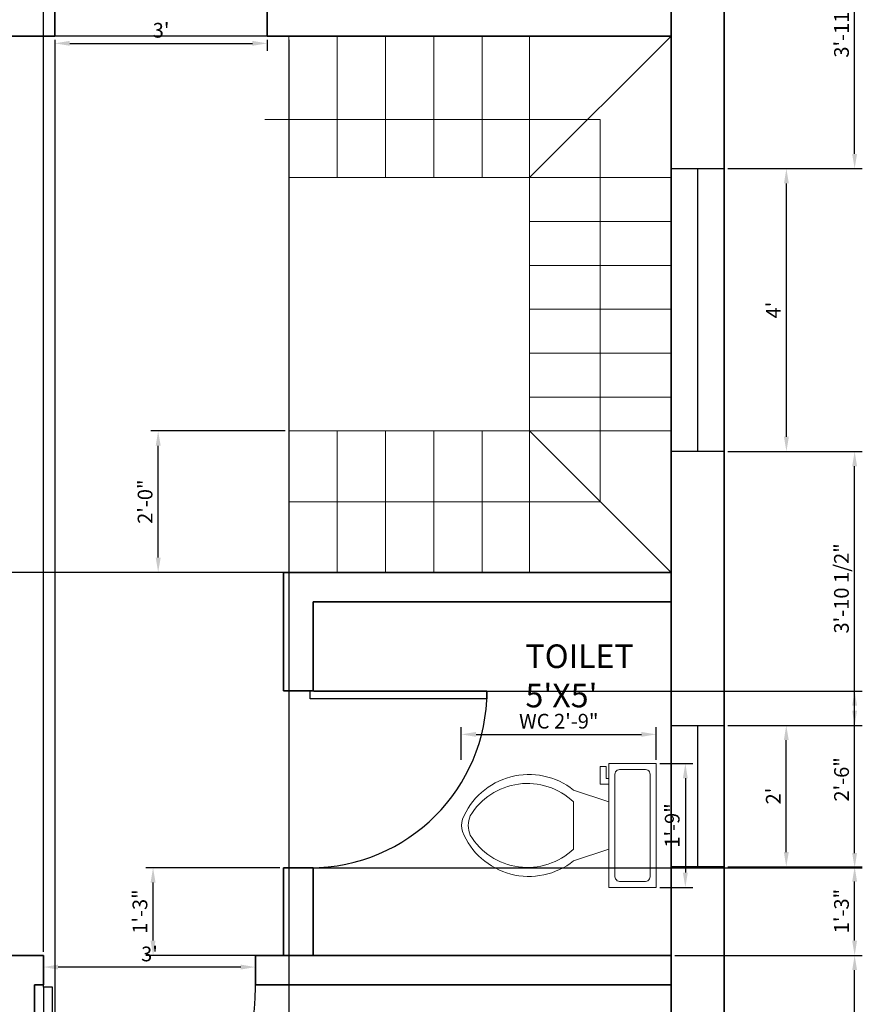
# Model space of a CAD drawing. Units: inches. Extents: x 2459 to 2755, y 1300 to 1776.
# Tile 3 of 4: x 2606 to 2750, y 1450 to 1617. Entities that reach past the tile are written whole.
import ezdxf

# ---------------------------------------------------------------- set-up
doc = ezdxf.new("R2010")
doc.units = ezdxf.units.IN
for name, color, linetype, lineweight in [('A-AREA-IDEN', 3, 'Continuous', 25), ('A-FLOR-FIXT', 8, 'Continuous', 18), ('A-FLOR-STRS', 7, 'Continuous', 18), ('A-WALL', 7, 'Continuous', 35), ('DIM', 4, 'Continuous', 18), ('DOOR', 20, 'Continuous', 25), ('WIN', 2, 'Continuous', 25)]:
    doc.layers.add(name, color=color, linetype=linetype, lineweight=lineweight)
doc.styles.get("Standard").update_dxf_attribs({"font": 'arial.ttf'})
doc.dimstyles.new('ISO-25', dxfattribs={"dimtxt": 2.5, "dimasz": 2.5, "dimexe": 1.25, "dimexo": 0.625, "dimtad": 1, "dimlunit": 3, "dimtxsty": 'Standard', "dimcen": 2.5, "dimadec": 0, "dimazin": 0, "dimtfac": 1, "dimtmove": 0, "dimatfit": 3, "dimfxl": 1, "dimarcsym": 0})

# ---------------------------------------------------------------- blocks, each defined once
blk = doc.blocks.new('*U2')
for p, q in [((0, 0), (0, -6)), ((40, 0), (40, -6))]:
    blk.add_line(p, q)
blk.add_lwpolyline([(0, 0), (0, 40), (1.75, 40), (1.75, 0)], close=True)
blk.add_arc((0, 0), 40, 0, 90)
blk = doc.blocks.new('*U5')
for p, q in [((0, 0), (0, 6)), ((40, 0), (40, 6))]:
    blk.add_line(p, q)
blk.add_lwpolyline([(0, 0), (0, -40), (1.75, -40), (1.75, 0)], close=True)
blk.add_arc((0, 0), 40, 270, 0)
blk = doc.blocks.new('Toilet - top')
for p, q in [((9.5, -6), (9.5, -2)), ((-8, -8.5), (-8, -8)), ((-7, -8), (-7, -9.5)), ((-4, -8), (-6, -14)), ((4, -8), (6, -14)), ((-10, -8.5), (-8, -8.5)), ((-10, -9.5), (-10, -8.5)), ((-7, -9.5), (-10, -9.5)), ((4, -14), (-4, -14))]:
    blk.add_line(p, q)
blk.add_lwpolyline([(10.5, -8), (10.5, 0), (-10.5, 0), (-10.5, -8)], close=True)
for points in [[(8.5, -1), (-8.5, -1)], [(-9.5, -2), (-9.5, -6)], [(-8.5, -7), (8.5, -7)]]:
    blk.add_lwpolyline(points)
for centre, radius, start, end in [((-8.62, -1.88), 0.884, 81.8699, 188.1301), ((8.62, -1.88), 0.884, 351.8699, 98.1301), ((-8.62, -6.12), 0.884, 171.8699, 278.1301), ((8.62, -6.12), 0.884, 261.8699, 8.1301), ((3.52, -21.58), 12.17, 141.4691, 247.9714), ((4.2, -21.82), 11.33, 136.3677, 238.9468), ((-3.52, -21.58), 12.17, 292.0284, 38.5307), ((-4.2, -21.82), 11.33, 301.053, 43.6321), ((0, -27.88), 4, 245.7318, 294.2682), ((0, -29), 4, 254.8605, 285.1395)]:
    blk.add_arc(centre, radius, start, end)
blk = doc.blocks.new('*D23')
at = {"layer": 'Defpoints', "color": 0, "transparency": 16777216}
for p in [(2612.48, 1614.32), (2648.48, 1614.32), (2648.48, 1613.1)]:
    blk.add_point(p, dxfattribs=at)
at = {"layer": 'DIM', "color": 0, "lineweight": -2, "transparency": 16777216}
for p, q in [((2612.48, 1613.69), (2612.48, 1611.85)), ((2614.98, 1613.1), (2645.98, 1613.1)), ((2648.48, 1613.69), (2648.48, 1611.85))]:
    blk.add_line(p, q, dxfattribs=at)
at = {"layer": 'DIM', "color": 0, "transparency": 16777216}
for points in [[(2614.98, 1613.52), (2614.98, 1612.69), (2612.48, 1613.1)], [(2645.98, 1613.52), (2645.98, 1612.69), (2648.48, 1613.1)]]:
    blk.add_solid(points, dxfattribs=at)
at = {"layer": 'DIM', "color": 0, "transparency": 16777216, "insert": (2630.48, 1615), "char_height": 2.5, "attachment_point": 5}
blk.add_mtext("3'", dxfattribs=at)
blk = doc.blocks.new('*D27')
at = {"layer": 'Defpoints', "color": 0, "transparency": 16777216}
for p in [(2726, 1497.36), (2736.55, 1497.36), (2726, 1473.36)]:
    blk.add_point(p, dxfattribs=at)
at = {"layer": 'DIM', "color": 0, "lineweight": -2, "transparency": 16777216}
for p, q in [((2726.62, 1497.36), (2737.8, 1497.36)), ((2736.55, 1475.86), (2736.55, 1494.86)), ((2726.62, 1473.36), (2737.8, 1473.36))]:
    blk.add_line(p, q, dxfattribs=at)
at = {"layer": 'DIM', "color": 0, "transparency": 16777216}
for points in [[(2736.14, 1494.86), (2736.97, 1494.86), (2736.55, 1497.36)], [(2736.14, 1475.86), (2736.97, 1475.86), (2736.55, 1473.36)]]:
    blk.add_solid(points, dxfattribs=at)
at = {"layer": 'DIM', "color": 0, "transparency": 16777216, "insert": (2734.67, 1485.36), "char_height": 2.5, "attachment_point": 5, "rotation": 90}
blk.add_mtext("2'", dxfattribs=at)
blk = doc.blocks.new('*D28')
at = {"layer": 'Defpoints', "color": 0, "transparency": 16777216}
for p in [(2726, 1591.84), (2736.57, 1591.84), (2726, 1543.84)]:
    blk.add_point(p, dxfattribs=at)
at = {"layer": 'DIM', "color": 0, "lineweight": -2, "transparency": 16777216}
for p, q in [((2726.62, 1591.84), (2737.82, 1591.84)), ((2736.57, 1546.34), (2736.57, 1589.34)), ((2726.62, 1543.84), (2737.82, 1543.84))]:
    blk.add_line(p, q, dxfattribs=at)
at = {"layer": 'DIM', "color": 0, "transparency": 16777216}
for points in [[(2736.16, 1589.34), (2736.99, 1589.34), (2736.57, 1591.84)], [(2736.16, 1546.34), (2736.99, 1546.34), (2736.57, 1543.84)]]:
    blk.add_solid(points, dxfattribs=at)
at = {"layer": 'DIM', "color": 0, "transparency": 16777216, "insert": (2734.7, 1567.84), "char_height": 2.5, "attachment_point": 5, "rotation": 90}
blk.add_mtext("4'", dxfattribs=at)
blk = doc.blocks.new('*D32')
at = {"layer": 'Defpoints', "color": 0, "transparency": 16777216}
for p in [(2610.51, 1458.32), (2646.51, 1458.32), (2610.51, 1456.34)]:
    blk.add_point(p, dxfattribs=at)
at = {"layer": 'DIM', "color": 0, "lineweight": -2, "transparency": 16777216}
for p, q in [((2610.51, 1457.69), (2610.51, 1455.09)), ((2646.51, 1457.69), (2646.51, 1455.09)), ((2644.01, 1456.34), (2613.01, 1456.34))]:
    blk.add_line(p, q, dxfattribs=at)
at = {"layer": 'DIM', "color": 0, "transparency": 16777216}
for points in [[(2613.01, 1456.75), (2613.01, 1455.92), (2610.51, 1456.34)], [(2644.01, 1456.75), (2644.01, 1455.92), (2646.51, 1456.34)]]:
    blk.add_solid(points, dxfattribs=at)
at = {"layer": 'DIM', "color": 0, "transparency": 16777216, "insert": (2628.51, 1458.24), "char_height": 2.5, "attachment_point": 5}
blk.add_mtext("3'", dxfattribs=at)
blk = doc.blocks.new('WIN-48IN')
blk.add_line((4.5, 48), (4.5, 0))
blk.add_lwpolyline([(0, 48), (9, 48), (9, 0), (0, 0)], close=True)
blk = doc.blocks.new('WIN-24IN')
blk.add_line((4.5, 24), (4.5, 0))
blk.add_lwpolyline([(0, 24), (9, 24), (9, 0), (0, 0)], close=True)
blk = doc.blocks.new('*D55')
at = {"layer": 'Defpoints', "color": 0, "transparency": 16777216}
for p in [(2714.47, 1495.83), (2681.42, 1490.87), (2714.47, 1490.87)]:
    blk.add_point(p, dxfattribs=at)
at = {"layer": 'DIM', "color": 0, "lineweight": -2, "transparency": 16777216}
for p, q in [((2681.42, 1491.49), (2681.42, 1497.08)), ((2683.92, 1495.83), (2711.97, 1495.83)), ((2714.47, 1491.49), (2714.47, 1497.08))]:
    blk.add_line(p, q, dxfattribs=at)
at = {"layer": 'DIM', "color": 0, "transparency": 16777216}
for points in [[(2683.92, 1496.24), (2683.92, 1495.41), (2681.42, 1495.83)], [(2711.97, 1496.24), (2711.97, 1495.41), (2714.47, 1495.83)]]:
    blk.add_solid(points, dxfattribs=at)
at = {"layer": 'DIM', "color": 0, "transparency": 16777216, "insert": (2697.95, 1497.74), "char_height": 2.5, "attachment_point": 5}
blk.add_mtext('WC 2\'-9"', dxfattribs=at)
blk = doc.blocks.new('*D56')
at = {"layer": 'Defpoints', "color": 0, "transparency": 16777216}
for p in [(2714.47, 1490.87), (2714.47, 1469.87), (2719.43, 1469.87)]:
    blk.add_point(p, dxfattribs=at)
at = {"layer": 'DIM', "color": 0, "lineweight": -2, "transparency": 16777216}
for p, q in [((2715.09, 1490.87), (2720.68, 1490.87)), ((2719.43, 1488.37), (2719.43, 1472.37)), ((2715.09, 1469.87), (2720.68, 1469.87))]:
    blk.add_line(p, q, dxfattribs=at)
at = {"layer": 'DIM', "color": 0, "transparency": 16777216}
for points in [[(2719.01, 1488.37), (2719.84, 1488.37), (2719.43, 1490.87)], [(2719.01, 1472.37), (2719.84, 1472.37), (2719.43, 1469.87)]]:
    blk.add_solid(points, dxfattribs=at)
at = {"layer": 'DIM', "color": 0, "transparency": 16777216, "insert": (2717.52, 1480.37), "char_height": 2.5, "attachment_point": 5, "rotation": 90}
blk.add_mtext('1\'-9"', dxfattribs=at)
blk = doc.blocks.new('*D66')
at = {"layer": 'Defpoints', "color": 0, "transparency": 16777216}
for p in [(2717, 1458.32), (2748.15, 1458.32), (2726, 1423.98)]:
    blk.add_point(p, dxfattribs=at)
at = {"layer": 'DIM', "color": 0, "lineweight": -2, "transparency": 16777216}
for p, q in [((2717.62, 1458.32), (2749.4, 1458.32)), ((2748.15, 1426.48), (2748.15, 1455.82)), ((2726.62, 1423.98), (2749.4, 1423.98))]:
    blk.add_line(p, q, dxfattribs=at)
at = {"layer": 'DIM', "color": 0, "transparency": 16777216}
for points in [[(2747.73, 1455.82), (2748.56, 1455.82), (2748.15, 1458.32)], [(2747.73, 1426.48), (2748.56, 1426.48), (2748.15, 1423.98)]]:
    blk.add_solid(points, dxfattribs=at)
at = {"layer": 'DIM', "color": 0, "transparency": 16777216, "insert": (2746.23, 1441.15), "char_height": 2.5, "attachment_point": 5, "rotation": 90}
blk.add_mtext('2\'-10 1/2"', dxfattribs=at)
blk = doc.blocks.new('*D67')
at = {"layer": 'Defpoints', "color": 0, "transparency": 16777216}
for p in [(2726, 1473.36), (2748.15, 1473.36), (2717, 1458.32)]:
    blk.add_point(p, dxfattribs=at)
at = {"layer": 'DIM', "color": 0, "lineweight": -2, "transparency": 16777216}
for p, q in [((2726.62, 1473.36), (2749.4, 1473.36)), ((2748.15, 1460.82), (2748.15, 1470.86)), ((2717.62, 1458.32), (2749.4, 1458.32))]:
    blk.add_line(p, q, dxfattribs=at)
at = {"layer": 'DIM', "color": 0, "transparency": 16777216}
for points in [[(2747.73, 1470.86), (2748.56, 1470.86), (2748.15, 1473.36)], [(2747.73, 1460.82), (2748.56, 1460.82), (2748.15, 1458.32)]]:
    blk.add_solid(points, dxfattribs=at)
at = {"layer": 'DIM', "color": 0, "transparency": 16777216, "insert": (2746.24, 1465.84), "char_height": 2.5, "attachment_point": 5, "rotation": 90}
blk.add_mtext('1\'-3"', dxfattribs=at)
blk = doc.blocks.new('*D68')
at = {"layer": 'Defpoints', "color": 0, "transparency": 16777216}
for p in [(2726, 1543.84), (2748.15, 1543.84), (2726, 1497.36)]:
    blk.add_point(p, dxfattribs=at)
at = {"layer": 'DIM', "color": 0, "lineweight": -2, "transparency": 16777216}
for p, q in [((2726.62, 1543.84), (2749.4, 1543.84)), ((2748.15, 1499.86), (2748.15, 1541.34)), ((2726.62, 1497.36), (2749.4, 1497.36))]:
    blk.add_line(p, q, dxfattribs=at)
at = {"layer": 'DIM', "color": 0, "transparency": 16777216}
for points in [[(2747.73, 1541.34), (2748.56, 1541.34), (2748.15, 1543.84)], [(2747.73, 1499.86), (2748.56, 1499.86), (2748.15, 1497.36)]]:
    blk.add_solid(points, dxfattribs=at)
at = {"layer": 'DIM', "color": 0, "transparency": 16777216, "insert": (2746.23, 1520.6), "char_height": 2.5, "attachment_point": 5, "rotation": 90}
blk.add_mtext('3\'-10 1/2"', dxfattribs=at)
blk = doc.blocks.new('*D69')
at = {"layer": 'Defpoints', "color": 0, "transparency": 16777216}
for p in [(2726, 1638.95), (2748.15, 1638.95), (2726, 1591.84)]:
    blk.add_point(p, dxfattribs=at)
at = {"layer": 'DIM', "color": 0, "lineweight": -2, "transparency": 16777216}
for p, q in [((2726.62, 1638.95), (2749.4, 1638.95)), ((2748.15, 1594.34), (2748.15, 1636.45)), ((2726.62, 1591.84), (2749.4, 1591.84))]:
    blk.add_line(p, q, dxfattribs=at)
at = {"layer": 'DIM', "color": 0, "transparency": 16777216}
for points in [[(2747.73, 1636.45), (2748.56, 1636.45), (2748.15, 1638.95)], [(2747.73, 1594.34), (2748.56, 1594.34), (2748.15, 1591.84)]]:
    blk.add_solid(points, dxfattribs=at)
at = {"layer": 'DIM', "color": 0, "transparency": 16777216, "insert": (2746.24, 1615.39), "char_height": 2.5, "attachment_point": 5, "rotation": 90}
blk.add_mtext('3\'-11"', dxfattribs=at)
blk = doc.blocks.new('*D71')
at = {"layer": 'Defpoints', "color": 0, "transparency": 16777216}
for p in [(2655.77, 1503.19), (2748.15, 1503.19), (2655.77, 1473.19)]:
    blk.add_point(p, dxfattribs=at)
at = {"layer": 'DIM', "color": 0, "lineweight": -2, "transparency": 16777216}
for p, q in [((2656.39, 1503.19), (2749.4, 1503.19)), ((2748.15, 1475.69), (2748.15, 1500.69)), ((2656.39, 1473.19), (2749.4, 1473.19))]:
    blk.add_line(p, q, dxfattribs=at)
at = {"layer": 'DIM', "color": 0, "transparency": 16777216}
for points in [[(2747.73, 1500.69), (2748.56, 1500.69), (2748.15, 1503.19)], [(2747.73, 1475.69), (2748.56, 1475.69), (2748.15, 1473.19)]]:
    blk.add_solid(points, dxfattribs=at)
at = {"layer": 'DIM', "color": 0, "transparency": 16777216, "insert": (2746.25, 1488.19), "char_height": 2.5, "attachment_point": 5, "rotation": 90}
blk.add_mtext('2\'-6"', dxfattribs=at)
blk = doc.blocks.new('*D72')
at = {"layer": 'Defpoints', "color": 0, "transparency": 16777216}
for p in [(2652.14, 1614.32), (2717, 1614.32), (2717, 1302.17)]:
    blk.add_point(p, dxfattribs=at)
at = {"layer": 'DIM', "color": 0, "lineweight": -2, "transparency": 16777216}
for p, q in [((2652.14, 1613.69), (2652.14, 1300.92)), ((2717, 1613.69), (2717, 1300.92)), ((2654.64, 1302.17), (2714.5, 1302.17))]:
    blk.add_line(p, q, dxfattribs=at)
at = {"layer": 'DIM', "color": 0, "transparency": 16777216}
for points in [[(2654.64, 1302.58), (2654.64, 1301.75), (2652.14, 1302.17)], [(2714.5, 1302.58), (2714.5, 1301.75), (2717, 1302.17)]]:
    blk.add_solid(points, dxfattribs=at)
at = {"layer": 'DIM', "color": 0, "transparency": 16777216, "insert": (2684.57, 1304.06), "char_height": 2.5, "attachment_point": 5}
blk.add_mtext('5\'-5"', dxfattribs=at)
blk = doc.blocks.new('*D73')
at = {"layer": 'Defpoints', "color": 0, "transparency": 16777216}
for p in [(2464.85, 1614.32), (2652.14, 1614.32), (2652.14, 1523.32)]:
    blk.add_point(p, dxfattribs=at)
at = {"layer": 'DIM', "color": 0, "lineweight": -2, "transparency": 16777216}
for p, q in [((2651.52, 1614.32), (2463.6, 1614.32)), ((2464.85, 1525.82), (2464.85, 1611.82)), ((2651.52, 1523.32), (2463.6, 1523.32))]:
    blk.add_line(p, q, dxfattribs=at)
at = {"layer": 'DIM', "color": 0, "transparency": 16777216}
for points in [[(2464.43, 1611.82), (2465.26, 1611.82), (2464.85, 1614.32)], [(2464.43, 1525.82), (2465.26, 1525.82), (2464.85, 1523.32)]]:
    blk.add_solid(points, dxfattribs=at)
at = {"layer": 'DIM', "color": 0, "transparency": 16777216, "insert": (2462.97, 1568.82), "char_height": 2.5, "attachment_point": 5, "rotation": 90}
blk.add_mtext('7\'-7"', dxfattribs=at)
blk = doc.blocks.new('*D74')
at = {"layer": 'Defpoints', "color": 0, "transparency": 16777216}
for p in [(2629.99, 1547.32), (2652.14, 1547.32), (2652.14, 1523.32)]:
    blk.add_point(p, dxfattribs=at)
at = {"layer": 'DIM', "color": 0, "lineweight": -2, "transparency": 16777216}
for p, q in [((2651.52, 1547.32), (2628.74, 1547.32)), ((2629.99, 1525.82), (2629.99, 1544.82)), ((2651.52, 1523.32), (2628.74, 1523.32))]:
    blk.add_line(p, q, dxfattribs=at)
at = {"layer": 'DIM', "color": 0, "transparency": 16777216}
for points in [[(2629.57, 1544.82), (2630.41, 1544.82), (2629.99, 1547.32)], [(2629.57, 1525.82), (2630.41, 1525.82), (2629.99, 1523.32)]]:
    blk.add_solid(points, dxfattribs=at)
at = {"layer": 'DIM', "color": 0, "transparency": 16777216, "insert": (2628.09, 1535.32), "char_height": 2.5, "attachment_point": 5, "rotation": 90}
blk.add_mtext('2\'-0"', dxfattribs=at)
blk = doc.blocks.new('*D76')
at = {"layer": 'Defpoints', "color": 0, "transparency": 16777216}
for p in [(2597, 1614.32), (2612.48, 1614.32), (2612.48, 1302.17)]:
    blk.add_point(p, dxfattribs=at)
at = {"layer": 'DIM', "color": 0, "lineweight": -2, "transparency": 16777216}
for p, q in [((2597, 1613.69), (2597, 1300.92)), ((2612.48, 1613.69), (2612.48, 1300.92)), ((2599.5, 1302.17), (2609.98, 1302.17))]:
    blk.add_line(p, q, dxfattribs=at)
at = {"layer": 'DIM', "color": 0, "transparency": 16777216}
for points in [[(2599.5, 1302.58), (2599.5, 1301.75), (2597, 1302.17)], [(2609.98, 1302.58), (2609.98, 1301.75), (2612.48, 1302.17)]]:
    blk.add_solid(points, dxfattribs=at)
at = {"layer": 'DIM', "color": 0, "transparency": 16777216, "insert": (2604.74, 1304.09), "char_height": 2.5, "attachment_point": 5}
blk.add_mtext('1\'-3 1/2"', dxfattribs=at)
blk = doc.blocks.new('*D78')
at = {"layer": 'Defpoints', "color": 0, "transparency": 16777216}
for p in [(2610.51, 1770.47), (2590.97, 1458.32), (2610.51, 1458.32)]:
    blk.add_point(p, dxfattribs=at)
at = {"layer": 'DIM', "color": 0, "lineweight": -2, "transparency": 16777216}
for p, q in [((2590.97, 1458.94), (2590.97, 1771.72)), ((2610.51, 1458.94), (2610.51, 1771.72)), ((2593.47, 1770.47), (2608.01, 1770.47))]:
    blk.add_line(p, q, dxfattribs=at)
at = {"layer": 'DIM', "color": 0, "transparency": 16777216}
for points in [[(2593.47, 1770.88), (2593.47, 1770.05), (2590.97, 1770.47)], [(2608.01, 1770.88), (2608.01, 1770.05), (2610.51, 1770.47)]]:
    blk.add_solid(points, dxfattribs=at)
at = {"layer": 'DIM', "color": 0, "transparency": 16777216, "insert": (2600.74, 1772.38), "char_height": 2.5, "attachment_point": 5}
blk.add_mtext('1\'-7 1/2"', dxfattribs=at)
blk = doc.blocks.new('*D83')
at = {"layer": 'Defpoints', "color": 0, "transparency": 16777216}
for p in [(2629.12, 1473.19), (2651.27, 1473.19), (2651.27, 1458.32)]:
    blk.add_point(p, dxfattribs=at)
at = {"layer": 'DIM', "color": 0, "lineweight": -2, "transparency": 16777216}
for p, q in [((2650.64, 1473.19), (2627.87, 1473.19)), ((2629.12, 1460.82), (2629.12, 1470.69)), ((2650.64, 1458.32), (2627.87, 1458.32))]:
    blk.add_line(p, q, dxfattribs=at)
at = {"layer": 'DIM', "color": 0, "transparency": 16777216}
for points in [[(2628.7, 1470.69), (2629.54, 1470.69), (2629.12, 1473.19)], [(2628.7, 1460.82), (2629.54, 1460.82), (2629.12, 1458.32)]]:
    blk.add_solid(points, dxfattribs=at)
at = {"layer": 'DIM', "color": 0, "transparency": 16777216, "insert": (2627.22, 1465.76), "char_height": 2.5, "attachment_point": 5, "rotation": 90}
blk.add_mtext('1\'-3"', dxfattribs=at)

msp = doc.modelspace()

# ---------------------------------------------------------------- linework, layer by layer
at = {"layer": 'A-FLOR-STRS'}
for p, q in [((2652.141, 1590.317), (2652.141, 1614.317)), ((2660.344, 1590.317), (2660.344, 1614.317)), ((2668.548, 1590.317), (2668.548, 1614.317)), ((2676.752, 1590.317), (2676.752, 1614.317)), ((2684.955, 1590.317), (2684.955, 1614.317)), ((2692.997, 1590.317), (2692.997, 1614.317)), ((2692.997, 1590.317), (2716.997, 1614.317)), ((2648.088, 1600.177), (2704.997, 1600.177)), ((2704.997, 1600.177), (2704.997, 1535.317)), ((2652.141, 1590.317), (2692.997, 1590.317)), ((2692.997, 1547.317), (2692.997, 1590.317)), ((2692.997, 1590.317), (2716.997, 1590.317)), ((2692.997, 1582.867), (2716.997, 1582.867)), ((2692.997, 1575.417), (2716.997, 1575.417)), ((2692.997, 1567.967), (2716.997, 1567.967)), ((2692.997, 1560.517), (2716.997, 1560.517)), ((2692.997, 1553.067), (2716.997, 1553.067)), ((2652.141, 1547.317), (2652.141, 1523.317)), ((2652.141, 1547.317), (2692.997, 1547.317)), ((2660.344, 1547.317), (2660.344, 1523.317)), ((2668.548, 1547.317), (2668.548, 1523.317)), ((2676.752, 1547.317), (2676.752, 1523.317)), ((2684.955, 1547.317), (2684.955, 1523.317)), ((2692.997, 1547.317), (2716.997, 1547.317)), ((2692.997, 1547.317), (2692.997, 1523.317)), ((2692.997, 1547.317), (2716.997, 1523.317)), ((2704.997, 1535.317), (2652.141, 1535.317))]:
    msp.add_line(p, q, dxfattribs=at)
at = {"layer": 'A-WALL'}
for p, q in [((2725.997, 1324.317), (2725.997, 1748.317)), ((2716.997, 1333.317), (2716.997, 1739.317)), ((2596.996, 1614.317), (2612.476, 1614.317)), ((2648.476, 1614.317), (2716.997, 1614.317)), ((2651.269, 1523.317), (2716.997, 1523.317)), ((2651.269, 1503.194), (2651.269, 1523.317)), ((2656.269, 1518.317), (2716.997, 1518.317)), ((2656.269, 1503.194), (2656.269, 1518.317)), ((2651.269, 1458.317), (2651.269, 1473.194)), ((2656.269, 1458.317), (2656.269, 1473.194)), ((2590.966, 1458.317), (2610.511, 1458.317)), ((2646.511, 1458.317), (2716.997, 1458.317)), ((2608.997, 1453.317), (2610.511, 1453.317)), ((2608.997, 1362.317), (2608.997, 1453.317)), ((2646.511, 1453.317), (2716.997, 1453.317))]:
    msp.add_line(p, q, dxfattribs=at)
for points in [[(2612.476, 1614.317), (2612.476, 1619.317)], [(2648.476, 1619.317), (2648.476, 1614.317)], [(2651.269, 1503.194), (2656.269, 1503.194)], [(2656.269, 1473.194), (2651.269, 1473.194)], [(2610.511, 1453.317), (2610.511, 1458.317)], [(2646.511, 1458.317), (2646.511, 1453.317)]]:
    msp.add_lwpolyline(points, dxfattribs=at)

# ---------------------------------------------------------------- block references
at = {"layer": 'A-FLOR-FIXT', "rotation": 270}
msp.add_blockref('Toilet - top', (2714.469, 1480.369), dxfattribs=at)
at = {"layer": 'DOOR', "xscale": 0.9, "yscale": 0.9, "zscale": 0.9}
for name, p in [('*U2', (2612.476, 1619.717)), ('*U5', (2610.511, 1452.917))]:
    msp.add_blockref(name, p, dxfattribs=at)
at = {"layer": 'DOOR', "xscale": 0.75, "yscale": 0.75, "zscale": 0.75, "rotation": 270}
msp.add_blockref('*U2', (2655.769, 1503.194), dxfattribs=at)
at = {"layer": 'WIN'}
for name, p in [('WIN-48IN', (2716.997, 1543.839)), ('WIN-24IN', (2716.997, 1473.36))]:
    msp.add_blockref(name, p, dxfattribs=at)

# ---------------------------------------------------------------- texts
at = {"layer": 'A-AREA-IDEN', "insert": (2692.307, 1511.088), "char_height": 4, "attachment_point": 1}
msp.add_mtext_dynamic_manual_height_columns("{TOILET\\P5'X5'}", width=133.04104, gutter_width=21.155, heights=[0], dxfattribs=at)

# ---------------------------------------------------------------- dimensions: what is measured, and where the dimension line sits
at = {"layer": 'DIM'}
for base, p1, p2, override, picture, middle in [((2610.511, 1770.467), (2590.966, 1458.317), (2610.511, 1458.317), {"dimdec": 1, "dimlfac": 1, "dimrnd": 0, "dimzin": 1, "dimdsep": 46, "dimlunit": 4, "dimfrac": 2}, '*D78', (2600.738, 1772.385)), ((2648.476, 1613.102), (2612.476, 1614.317), (2648.476, 1614.317), {"dimclrd": 0, "dimclre": 0, "dimclrt": 0}, '*D23', (2630.476, 1615.004)), ((2612.476, 1302.167), (2596.996, 1614.317), (2612.476, 1614.317), {"dimdec": 1, "dimlfac": 1, "dimrnd": 0, "dimzin": 1, "dimdsep": 46, "dimlunit": 4, "dimfrac": 2}, '*D76', (2604.736, 1304.086)), ((2716.997, 1302.167), (2652.141, 1614.317), (2716.997, 1614.317), {"dimdec": 1, "dimlfac": 1, "dimrnd": 0, "dimzin": 1, "dimdsep": 46, "dimlunit": 4, "dimfrac": 2}, '*D72', (2684.569, 1304.063)), ((2610.511, 1456.337), (2646.511, 1458.317), (2610.511, 1458.317), {"dimclrd": 0, "dimclre": 0, "dimclrt": 0}, '*D32', (2628.511, 1458.239))]:
    dim = msp.add_linear_dim(base=base, p1=p1, p2=p2, dimstyle='ISO-25', override=override, dxfattribs=at)
    dim.commit()
    dim.dimension.update_dxf_attribs({"geometry": picture, "text_midpoint": middle})
for base, p1, p2, angle, override, picture, middle in [((2748.147, 1638.951), (2725.997, 1591.839), (2725.997, 1638.951), 90, {"dimdec": 1, "dimlfac": 1, "dimrnd": 0, "dimzin": 1, "dimdsep": 46, "dimlunit": 4, "dimfrac": 2}, '*D69', (2746.245, 1615.395)), ((2464.847, 1614.317), (2652.141, 1523.317), (2652.141, 1614.317), 90, {"dimdec": 1, "dimlfac": 1, "dimrnd": 0, "dimzin": 1, "dimdsep": 46, "dimlunit": 4, "dimfrac": 2}, '*D73', (2462.972, 1568.817)), ((2736.574, 1591.839), (2725.997, 1543.839), (2725.997, 1591.839), 90, {"dimclrd": 0, "dimclre": 0, "dimclrt": 0}, '*D28', (2734.699, 1567.839)), ((2629.991, 1547.317), (2652.141, 1523.317), (2652.141, 1547.317), 90, {"dimdec": 1, "dimlfac": 1, "dimrnd": 0, "dimzin": 1, "dimdsep": 46, "dimlunit": 4, "dimfrac": 2}, '*D74', (2628.089, 1535.317)), ((2748.147, 1543.839), (2725.997, 1497.36), (2725.997, 1543.839), 90, {"dimdec": 1, "dimlfac": 1, "dimrnd": 0, "dimzin": 1, "dimdsep": 46, "dimlunit": 4, "dimfrac": 2}, '*D68', (2746.228, 1520.6)), ((2748.147, 1503.194), (2655.769, 1473.194), (2655.769, 1503.194), 90, {"dimdec": 1, "dimlfac": 1, "dimrnd": 0, "dimzin": 1, "dimdsep": 46, "dimlunit": 4, "dimfrac": 2}, '*D71', (2746.245, 1488.194)), ((2736.554, 1497.36), (2725.997, 1473.36), (2725.997, 1497.36), 90, {"dimclrd": 0, "dimclre": 0, "dimclrt": 0}, '*D27', (2734.674, 1485.36)), ((2719.426, 1469.869), (2714.469, 1490.869), (2714.469, 1469.869), 270, {"dimdec": 1, "dimlfac": 1, "dimrnd": 0, "dimzin": 1, "dimdsep": 46, "dimlunit": 4, "dimfrac": 2}, '*D56', (2717.524, 1480.369)), ((2629.119, 1473.194), (2651.269, 1458.317), (2651.269, 1473.194), 90, {"dimdec": 1, "dimlfac": 1, "dimrnd": 0, "dimzin": 1, "dimdsep": 46, "dimlunit": 4, "dimfrac": 2}, '*D83', (2627.217, 1465.755)), ((2748.147, 1473.36), (2716.997, 1458.317), (2725.997, 1473.36), 90, {"dimdec": 1, "dimlfac": 1, "dimrnd": 0, "dimzin": 1, "dimdsep": 46, "dimlunit": 4, "dimfrac": 2}, '*D67', (2746.245, 1465.839)), ((2748.147, 1458.317), (2725.997, 1423.984), (2716.997, 1458.317), 90, {"dimdec": 1, "dimlfac": 1, "dimrnd": 0, "dimzin": 1, "dimdsep": 46, "dimlunit": 4, "dimfrac": 2}, '*D66', (2746.229, 1441.151))]:
    dim = msp.add_linear_dim(base=base, p1=p1, p2=p2, angle=angle, dimstyle='ISO-25', override=override, dxfattribs=at)
    dim.commit()
    dim.dimension.update_dxf_attribs({"geometry": picture, "text_midpoint": middle})
dim = msp.add_linear_dim(base=(2714.469, 1495.826), p1=(2681.423, 1490.869), p2=(2714.469, 1490.869), text='WC <>', dimstyle='ISO-25', override={"dimdec": 1, "dimlfac": 1, "dimrnd": 0, "dimzin": 1, "dimdsep": 46, "dimlunit": 4, "dimfrac": 2}, dxfattribs=at)
dim.commit()
dim.dimension.update_dxf_attribs({"geometry": '*D55', "text_midpoint": (2697.946, 1497.743)})

doc.saveas('drawing.dxf')
